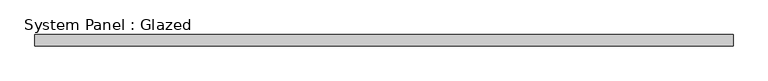
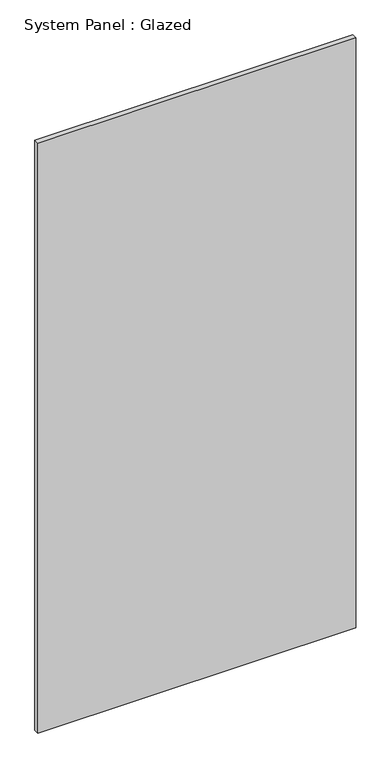
"""IFC4 building model written with IfcOpenShell, lengths in millimetres: plate geometry, System Panel : Glazed."""

from ifc_helpers import new_model, si_unit, origin, origin_with_axes, place, context, project, spatial, polyline, outline, extrude, source, transform, mapped, element, save


def system_panel_glazed_94d7f8cb(model_context):
    return source(origin(), model_context, "Body", "SweptSolid", [
        extrude(outline(polyline([(764.032, 24.5), (-764.032, 24.5), (-764.032, 49.5), (764.032, 49.5), (764.032, 24.5)])), origin_with_axes(), (0.0, 0.0, 1.0), 3000.0),
    ])


if __name__ == "__main__":
    model = new_model("IFC4")
    model_context = context("Model", 3, world=origin())
    ifc_project = project(units=[si_unit("LENGTHUNIT", "METRE", prefix="MILLI")], contexts=[model_context])
    site = spatial("IfcSite", under=ifc_project)
    building = spatial("IfcBuilding", under=site)
    placement = place(None, origin())
    system_panel_glazed_shape = system_panel_glazed_94d7f8cb(model_context)
    element("IfcPlate", 1, ObjectType="System Panel : Glazed", at=placement, inside=building, context=model_context, shape_type="MappedRepresentation", body=[
        mapped(system_panel_glazed_shape, transform((0.0, 0.0, 0.0), x_axis=(1.0, 0.0, 0.0), y_axis=(0.0, 1.0, 0.0), z_axis=(0.0, 0.0, 1.0))),
    ])
    save(model, "model.ifc")

# Revit data of these elements
# Type "System Panel : Glazed"
#   Keynote = "H11"
#   Construction Type Id = "GSP4R"
#   Analytic Construction = "1/8 in Pilkington single glazing"
#   Visual Light Transmittance = 0.9
#   Solar Heat Gain Coefficient = 0.86
#   Heat Transfer Coefficient (U) = 6.7069 W/(m²·K)
#   Define Thermal Properties by = 1
# Element 1 (IfcPlate, "System Panel : Glazed")
#   Materials on its faces: "Glass"
# Materials
#   "Glass": class "Glass", colour RGB 0 128 192, transparency 0.9, Description = "Soda Lime Glass", Cost = 0
